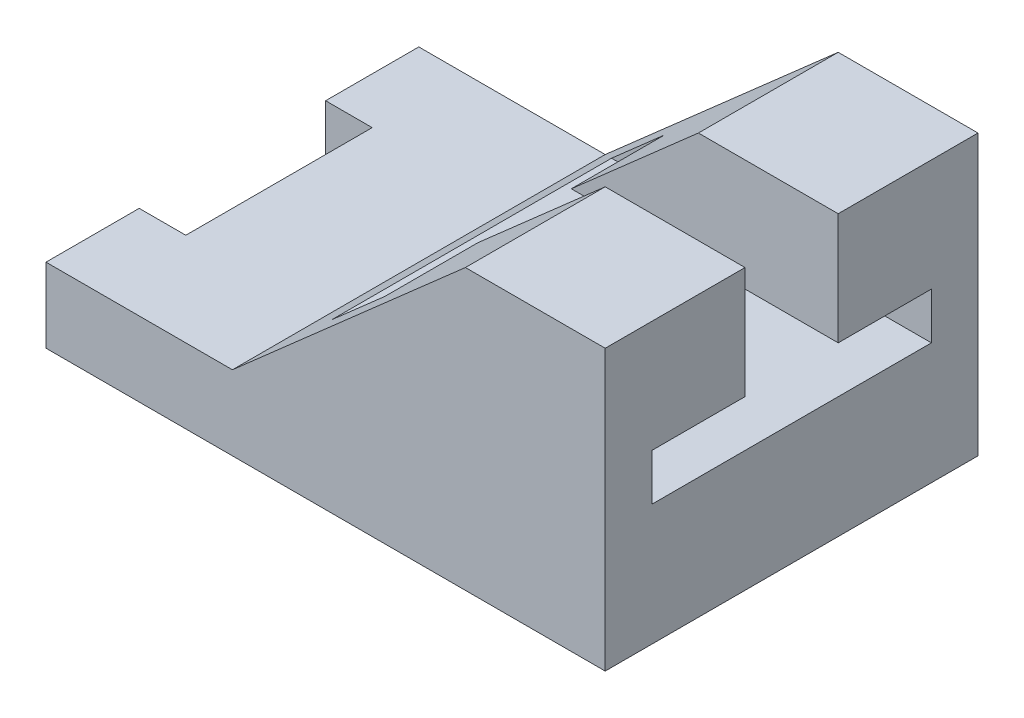
ISO-10303-21;
HEADER;
FILE_DESCRIPTION(('STEP AP214'),'2;1');
FILE_NAME('part.step','',(''),(''),'','','');
FILE_SCHEMA(('AUTOMOTIVE_DESIGN { 1 0 10303 214 1 1 1 1 }'));
ENDSEC;
DATA;
#1=APPLICATION_CONTEXT('core data for automotive mechanical design processes');
#2=APPLICATION_PROTOCOL_DEFINITION('international standard','automotive_design',2000,#1);
#3=PRODUCT_CONTEXT('',#1,'mechanical');
#4=PRODUCT('Part','Part','',(#3));
#5=PRODUCT_RELATED_PRODUCT_CATEGORY('part','',(#4));
#6=PRODUCT_DEFINITION_FORMATION('','',#4);
#7=PRODUCT_DEFINITION_CONTEXT('part definition',#1,'design');
#8=PRODUCT_DEFINITION('design','',#6,#7);
#9=PRODUCT_DEFINITION_SHAPE('','',#8);
#10=(LENGTH_UNIT() NAMED_UNIT(*) SI_UNIT(.MILLI.,.METRE.));
#11=(NAMED_UNIT(*) PLANE_ANGLE_UNIT() SI_UNIT($,.RADIAN.));
#12=(NAMED_UNIT(*) SI_UNIT($,.STERADIAN.) SOLID_ANGLE_UNIT());
#13=UNCERTAINTY_MEASURE_WITH_UNIT(LENGTH_MEASURE(1.E-05),#10,'distance_accuracy_value','');
#14=(GEOMETRIC_REPRESENTATION_CONTEXT(3) GLOBAL_UNCERTAINTY_ASSIGNED_CONTEXT((#13)) GLOBAL_UNIT_ASSIGNED_CONTEXT((#10,
#11,#12)) REPRESENTATION_CONTEXT('',''));
#15=CARTESIAN_POINT('',(0.,0.,0.));
#16=DIRECTION('',(0.,0.,1.));
#17=DIRECTION('',(1.,0.,0.));
#18=AXIS2_PLACEMENT_3D('',#15,#16,#17);
#19=CARTESIAN_POINT('',(60.,30.,40.));
#20=DIRECTION('',(0.,-1.,0.));
#21=DIRECTION('',(0.,0.,-1.));
#22=AXIS2_PLACEMENT_3D('',#19,#20,#21);
#23=PLANE('',#22);
#24=DIRECTION('',(0.,0.,-1.));
#25=VECTOR('',#24,1.);
#26=CARTESIAN_POINT('',(45.,30.,40.));
#27=LINE('',#26,#25);
#28=CARTESIAN_POINT('',(45.,30.,15.));
#29=VERTEX_POINT('',#28);
#30=CARTESIAN_POINT('',(45.,30.,0.));
#31=VERTEX_POINT('',#30);
#32=EDGE_CURVE('E302',#29,#31,#27,.T.);
#33=ORIENTED_EDGE('',*,*,#32,.F.);
#34=DIRECTION('',(1.,0.,0.));
#35=VECTOR('',#34,1.);
#36=CARTESIAN_POINT('',(20.,30.,15.));
#37=LINE('',#36,#35);
#38=CARTESIAN_POINT('',(60.,30.,15.));
#39=VERTEX_POINT('',#38);
#40=EDGE_CURVE('E240',#29,#39,#37,.T.);
#41=ORIENTED_EDGE('',*,*,#40,.T.);
#42=DIRECTION('',(0.,0.,-1.));
#43=VECTOR('',#42,1.);
#44=CARTESIAN_POINT('',(60.,30.,40.));
#45=LINE('',#44,#43);
#46=CARTESIAN_POINT('',(60.,30.,0.));
#47=VERTEX_POINT('',#46);
#48=EDGE_CURVE('E194',#39,#47,#45,.T.);
#49=ORIENTED_EDGE('',*,*,#48,.T.);
#50=DIRECTION('',(-1.,0.,0.));
#51=VECTOR('',#50,1.);
#52=CARTESIAN_POINT('',(60.,30.,0.));
#53=LINE('',#52,#51);
#54=EDGE_CURVE('E292',#47,#31,#53,.T.);
#55=ORIENTED_EDGE('',*,*,#54,.T.);
#56=EDGE_LOOP('',(#33,#41,#49,#55));
#57=FACE_BOUND('',#56,.T.);
#58=ADVANCED_FACE('F43',(#57),#23,.F.);
#59=CARTESIAN_POINT('',(0.,0.,40.));
#60=DIRECTION('',(1.,0.,0.));
#61=DIRECTION('',(0.,0.,-1.));
#62=AXIS2_PLACEMENT_3D('',#59,#60,#61);
#63=PLANE('',#62);
#64=DIRECTION('',(0.,0.,-1.));
#65=VECTOR('',#64,1.);
#66=CARTESIAN_POINT('',(0.,8.,40.));
#67=LINE('',#66,#65);
#68=CARTESIAN_POINT('',(0.,8.,40.));
#69=VERTEX_POINT('',#68);
#70=CARTESIAN_POINT('',(0.,8.,30.));
#71=VERTEX_POINT('',#70);
#72=EDGE_CURVE('E297',#69,#71,#67,.T.);
#73=ORIENTED_EDGE('',*,*,#72,.T.);
#74=DIRECTION('',(0.,1.,0.));
#75=VECTOR('',#74,1.);
#76=CARTESIAN_POINT('',(0.,0.,30.));
#77=LINE('',#76,#75);
#78=CARTESIAN_POINT('',(0.,0.,30.));
#79=VERTEX_POINT('',#78);
#80=EDGE_CURVE('E250',#79,#71,#77,.T.);
#81=ORIENTED_EDGE('',*,*,#80,.F.);
#82=DIRECTION('',(0.,0.,-1.));
#83=VECTOR('',#82,1.);
#84=CARTESIAN_POINT('',(0.,0.,40.));
#85=LINE('',#84,#83);
#86=CARTESIAN_POINT('',(0.,0.,40.));
#87=VERTEX_POINT('',#86);
#88=EDGE_CURVE('E205',#87,#79,#85,.T.);
#89=ORIENTED_EDGE('',*,*,#88,.F.);
#90=DIRECTION('',(0.,-1.,0.));
#91=VECTOR('',#90,1.);
#92=CARTESIAN_POINT('',(0.,0.,40.));
#93=LINE('',#92,#91);
#94=EDGE_CURVE('E269',#69,#87,#93,.T.);
#95=ORIENTED_EDGE('',*,*,#94,.F.);
#96=EDGE_LOOP('',(#73,#81,#89,#95));
#97=FACE_BOUND('',#96,.T.);
#98=ADVANCED_FACE('F352',(#97),#63,.F.);
#99=CARTESIAN_POINT('',(0.,0.,10.));
#100=VERTEX_POINT('',#99);
#101=CARTESIAN_POINT('',(0.,0.,0.));
#102=VERTEX_POINT('',#101);
#103=EDGE_CURVE('E198',#100,#102,#85,.T.);
#104=ORIENTED_EDGE('',*,*,#103,.F.);
#105=DIRECTION('',(0.,-1.,0.));
#106=VECTOR('',#105,1.);
#107=CARTESIAN_POINT('',(0.,8.,10.));
#108=LINE('',#107,#106);
#109=CARTESIAN_POINT('',(0.,8.,10.));
#110=VERTEX_POINT('',#109);
#111=EDGE_CURVE('E260',#110,#100,#108,.T.);
#112=ORIENTED_EDGE('',*,*,#111,.F.);
#113=CARTESIAN_POINT('',(0.,8.,0.));
#114=VERTEX_POINT('',#113);
#115=EDGE_CURVE('E282',#110,#114,#67,.T.);
#116=ORIENTED_EDGE('',*,*,#115,.T.);
#117=DIRECTION('',(0.,-1.,0.));
#118=VECTOR('',#117,1.);
#119=CARTESIAN_POINT('',(0.,0.,0.));
#120=LINE('',#119,#118);
#121=EDGE_CURVE('E263',#114,#102,#120,.T.);
#122=ORIENTED_EDGE('',*,*,#121,.T.);
#123=EDGE_LOOP('',(#104,#112,#116,#122));
#124=FACE_BOUND('',#123,.T.);
#125=ADVANCED_FACE('F44',(#124),#63,.F.);
#126=CARTESIAN_POINT('',(0.,0.,40.));
#127=DIRECTION('',(0.,1.,0.));
#128=DIRECTION('',(0.,0.,1.));
#129=AXIS2_PLACEMENT_3D('',#126,#127,#128);
#130=PLANE('',#129);
#131=ORIENTED_EDGE('',*,*,#88,.T.);
#132=DIRECTION('',(-1.,0.,0.));
#133=VECTOR('',#132,1.);
#134=CARTESIAN_POINT('',(5.,0.,30.));
#135=LINE('',#134,#133);
#136=CARTESIAN_POINT('',(5.,0.,30.));
#137=VERTEX_POINT('',#136);
#138=EDGE_CURVE('E262',#137,#79,#135,.T.);
#139=ORIENTED_EDGE('',*,*,#138,.F.);
#140=DIRECTION('',(0.,0.,1.));
#141=VECTOR('',#140,1.);
#142=CARTESIAN_POINT('',(5.,0.,10.));
#143=LINE('',#142,#141);
#144=CARTESIAN_POINT('',(5.,0.,10.));
#145=VERTEX_POINT('',#144);
#146=EDGE_CURVE('E251',#145,#137,#143,.T.);
#147=ORIENTED_EDGE('',*,*,#146,.F.);
#148=DIRECTION('',(-1.,0.,0.));
#149=VECTOR('',#148,1.);
#150=CARTESIAN_POINT('',(5.,0.,10.));
#151=LINE('',#150,#149);
#152=EDGE_CURVE('E266',#145,#100,#151,.T.);
#153=ORIENTED_EDGE('',*,*,#152,.T.);
#154=ORIENTED_EDGE('',*,*,#103,.T.);
#155=DIRECTION('',(1.,0.,0.));
#156=VECTOR('',#155,1.);
#157=CARTESIAN_POINT('',(0.,0.,0.));
#158=LINE('',#157,#156);
#159=CARTESIAN_POINT('',(60.,0.,0.));
#160=VERTEX_POINT('',#159);
#161=EDGE_CURVE('E286',#102,#160,#158,.T.);
#162=ORIENTED_EDGE('',*,*,#161,.T.);
#163=DIRECTION('',(0.,0.,-1.));
#164=VECTOR('',#163,1.);
#165=CARTESIAN_POINT('',(60.,0.,40.));
#166=LINE('',#165,#164);
#167=CARTESIAN_POINT('',(60.,0.,40.));
#168=VERTEX_POINT('',#167);
#169=EDGE_CURVE('E192',#168,#160,#166,.T.);
#170=ORIENTED_EDGE('',*,*,#169,.F.);
#171=DIRECTION('',(1.,0.,0.));
#172=VECTOR('',#171,1.);
#173=CARTESIAN_POINT('',(0.,0.,40.));
#174=LINE('',#173,#172);
#175=EDGE_CURVE('E272',#87,#168,#174,.T.);
#176=ORIENTED_EDGE('',*,*,#175,.F.);
#177=EDGE_LOOP('',(#131,#139,#147,#153,#154,#162,#170,#176));
#178=FACE_BOUND('',#177,.T.);
#179=ADVANCED_FACE('F370',(#178),#130,.F.);
#180=CARTESIAN_POINT('',(60.,0.,40.));
#181=DIRECTION('',(-1.,0.,0.));
#182=DIRECTION('',(0.,0.,1.));
#183=AXIS2_PLACEMENT_3D('',#180,#181,#182);
#184=PLANE('',#183);
#185=ORIENTED_EDGE('',*,*,#48,.F.);
#186=DIRECTION('',(0.,1.,0.));
#187=VECTOR('',#186,1.);
#188=CARTESIAN_POINT('',(60.,30.,15.));
#189=LINE('',#188,#187);
#190=CARTESIAN_POINT('',(60.,18.,15.));
#191=VERTEX_POINT('',#190);
#192=EDGE_CURVE('E177',#191,#39,#189,.T.);
#193=ORIENTED_EDGE('',*,*,#192,.F.);
#194=DIRECTION('',(0.,0.,1.));
#195=VECTOR('',#194,1.);
#196=CARTESIAN_POINT('',(60.,18.,15.));
#197=LINE('',#196,#195);
#198=CARTESIAN_POINT('',(60.,18.,5.));
#199=VERTEX_POINT('',#198);
#200=EDGE_CURVE('E323',#199,#191,#197,.T.);
#201=ORIENTED_EDGE('',*,*,#200,.F.);
#202=DIRECTION('',(0.,1.,0.));
#203=VECTOR('',#202,1.);
#204=CARTESIAN_POINT('',(60.,18.,5.));
#205=LINE('',#204,#203);
#206=CARTESIAN_POINT('',(60.,13.,5.));
#207=VERTEX_POINT('',#206);
#208=EDGE_CURVE('E234',#207,#199,#205,.T.);
#209=ORIENTED_EDGE('',*,*,#208,.F.);
#210=DIRECTION('',(0.,0.,-1.));
#211=VECTOR('',#210,1.);
#212=CARTESIAN_POINT('',(60.,13.,5.));
#213=LINE('',#212,#211);
#214=CARTESIAN_POINT('',(60.,13.,35.));
#215=VERTEX_POINT('',#214);
#216=EDGE_CURVE('E328',#215,#207,#213,.T.);
#217=ORIENTED_EDGE('',*,*,#216,.F.);
#218=DIRECTION('',(0.,-1.,0.));
#219=VECTOR('',#218,1.);
#220=CARTESIAN_POINT('',(60.,13.,35.));
#221=LINE('',#220,#219);
#222=CARTESIAN_POINT('',(60.,18.,35.));
#223=VERTEX_POINT('',#222);
#224=EDGE_CURVE('E335',#223,#215,#221,.T.);
#225=ORIENTED_EDGE('',*,*,#224,.F.);
#226=DIRECTION('',(0.,0.,1.));
#227=VECTOR('',#226,1.);
#228=CARTESIAN_POINT('',(60.,18.,35.));
#229=LINE('',#228,#227);
#230=CARTESIAN_POINT('',(60.,18.,25.));
#231=VERTEX_POINT('',#230);
#232=EDGE_CURVE('E187',#231,#223,#229,.T.);
#233=ORIENTED_EDGE('',*,*,#232,.F.);
#234=DIRECTION('',(0.,-1.,0.));
#235=VECTOR('',#234,1.);
#236=CARTESIAN_POINT('',(60.,30.,25.));
#237=LINE('',#236,#235);
#238=CARTESIAN_POINT('',(60.,30.,25.));
#239=VERTEX_POINT('',#238);
#240=EDGE_CURVE('E166',#239,#231,#237,.T.);
#241=ORIENTED_EDGE('',*,*,#240,.F.);
#242=CARTESIAN_POINT('',(60.,30.,40.));
#243=VERTEX_POINT('',#242);
#244=EDGE_CURVE('E184',#243,#239,#45,.T.);
#245=ORIENTED_EDGE('',*,*,#244,.F.);
#246=DIRECTION('',(0.,1.,0.));
#247=VECTOR('',#246,1.);
#248=CARTESIAN_POINT('',(60.,0.,40.));
#249=LINE('',#248,#247);
#250=EDGE_CURVE('E277',#168,#243,#249,.T.);
#251=ORIENTED_EDGE('',*,*,#250,.F.);
#252=ORIENTED_EDGE('',*,*,#169,.T.);
#253=DIRECTION('',(0.,1.,0.));
#254=VECTOR('',#253,1.);
#255=CARTESIAN_POINT('',(60.,0.,0.));
#256=LINE('',#255,#254);
#257=EDGE_CURVE('E289',#160,#47,#256,.T.);
#258=ORIENTED_EDGE('',*,*,#257,.T.);
#259=EDGE_LOOP('',(#185,#193,#201,#209,#217,#225,#233,#241,#245,#251,#252,#258));
#260=FACE_BOUND('',#259,.T.);
#261=ADVANCED_FACE('F185',(#260),#184,.F.);
#262=ORIENTED_EDGE('',*,*,#244,.T.);
#263=DIRECTION('',(1.,0.,0.));
#264=VECTOR('',#263,1.);
#265=CARTESIAN_POINT('',(20.,30.,25.));
#266=LINE('',#265,#264);
#267=CARTESIAN_POINT('',(45.,30.,25.));
#268=VERTEX_POINT('',#267);
#269=EDGE_CURVE('E167',#268,#239,#266,.T.);
#270=ORIENTED_EDGE('',*,*,#269,.F.);
#271=CARTESIAN_POINT('',(45.,30.,40.));
#272=VERTEX_POINT('',#271);
#273=EDGE_CURVE('E196',#272,#268,#27,.T.);
#274=ORIENTED_EDGE('',*,*,#273,.F.);
#275=DIRECTION('',(-1.,0.,0.));
#276=VECTOR('',#275,1.);
#277=CARTESIAN_POINT('',(60.,30.,40.));
#278=LINE('',#277,#276);
#279=EDGE_CURVE('E191',#243,#272,#278,.T.);
#280=ORIENTED_EDGE('',*,*,#279,.F.);
#281=EDGE_LOOP('',(#262,#270,#274,#280));
#282=FACE_BOUND('',#281,.T.);
#283=ADVANCED_FACE('F186',(#282),#23,.F.);
#284=CARTESIAN_POINT('',(20.,8.,40.));
#285=DIRECTION('',(0.660627894892025,-0.750713516922755,0.));
#286=DIRECTION('',(0.750713516922755,0.660627894892025,0.));
#287=AXIS2_PLACEMENT_3D('',#284,#285,#286);
#288=PLANE('',#287);
#289=DIRECTION('',(0.,0.,1.));
#290=VECTOR('',#289,1.);
#291=CARTESIAN_POINT('',(31.3636363636364,18.,40.));
#292=LINE('',#291,#290);
#293=CARTESIAN_POINT('',(31.3636363636364,18.,5.));
#294=VERTEX_POINT('',#293);
#295=CARTESIAN_POINT('',(31.3636363636364,18.,15.));
#296=VERTEX_POINT('',#295);
#297=EDGE_CURVE('E51',#294,#296,#292,.T.);
#298=ORIENTED_EDGE('',*,*,#297,.T.);
#299=DIRECTION('',(0.750713516922755,0.660627894892025,0.));
#300=VECTOR('',#299,1.);
#301=CARTESIAN_POINT('',(20.,8.,15.));
#302=LINE('',#301,#300);
#303=EDGE_CURVE('E11',#296,#29,#302,.T.);
#304=ORIENTED_EDGE('',*,*,#303,.T.);
#305=ORIENTED_EDGE('',*,*,#32,.T.);
#306=DIRECTION('',(-0.750713516922755,-0.660627894892025,0.));
#307=VECTOR('',#306,1.);
#308=CARTESIAN_POINT('',(20.,8.,0.));
#309=LINE('',#308,#307);
#310=CARTESIAN_POINT('',(20.,8.,0.));
#311=VERTEX_POINT('',#310);
#312=EDGE_CURVE('E294',#31,#311,#309,.T.);
#313=ORIENTED_EDGE('',*,*,#312,.T.);
#314=DIRECTION('',(0.,0.,-1.));
#315=VECTOR('',#314,1.);
#316=CARTESIAN_POINT('',(20.,8.,40.));
#317=LINE('',#316,#315);
#318=CARTESIAN_POINT('',(20.,8.,40.));
#319=VERTEX_POINT('',#318);
#320=EDGE_CURVE('E296',#319,#311,#317,.T.);
#321=ORIENTED_EDGE('',*,*,#320,.F.);
#322=DIRECTION('',(-0.750713516922755,-0.660627894892025,0.));
#323=VECTOR('',#322,1.);
#324=CARTESIAN_POINT('',(20.,8.,40.));
#325=LINE('',#324,#323);
#326=EDGE_CURVE('E276',#272,#319,#325,.T.);
#327=ORIENTED_EDGE('',*,*,#326,.F.);
#328=ORIENTED_EDGE('',*,*,#273,.T.);
#329=DIRECTION('',(-0.750713516922755,-0.660627894892025,0.));
#330=VECTOR('',#329,1.);
#331=CARTESIAN_POINT('',(20.,8.,25.));
#332=LINE('',#331,#330);
#333=CARTESIAN_POINT('',(31.3636363636364,18.,25.));
#334=VERTEX_POINT('',#333);
#335=EDGE_CURVE('E174',#268,#334,#332,.T.);
#336=ORIENTED_EDGE('',*,*,#335,.T.);
#337=DIRECTION('',(0.,0.,1.));
#338=VECTOR('',#337,1.);
#339=CARTESIAN_POINT('',(31.3636363636364,18.,40.));
#340=LINE('',#339,#338);
#341=CARTESIAN_POINT('',(31.3636363636364,18.,35.));
#342=VERTEX_POINT('',#341);
#343=EDGE_CURVE('E206',#334,#342,#340,.T.);
#344=ORIENTED_EDGE('',*,*,#343,.T.);
#345=DIRECTION('',(-0.750713516922755,-0.660627894892025,0.));
#346=VECTOR('',#345,1.);
#347=CARTESIAN_POINT('',(20.,8.,35.));
#348=LINE('',#347,#346);
#349=CARTESIAN_POINT('',(25.6818181818182,13.,35.));
#350=VERTEX_POINT('',#349);
#351=EDGE_CURVE('E207',#342,#350,#348,.T.);
#352=ORIENTED_EDGE('',*,*,#351,.T.);
#353=DIRECTION('',(0.,0.,-1.));
#354=VECTOR('',#353,1.);
#355=CARTESIAN_POINT('',(25.6818181818182,13.,40.));
#356=LINE('',#355,#354);
#357=CARTESIAN_POINT('',(25.6818181818182,13.,5.));
#358=VERTEX_POINT('',#357);
#359=EDGE_CURVE('E215',#350,#358,#356,.T.);
#360=ORIENTED_EDGE('',*,*,#359,.T.);
#361=DIRECTION('',(0.750713516922755,0.660627894892025,0.));
#362=VECTOR('',#361,1.);
#363=CARTESIAN_POINT('',(20.,8.,5.));
#364=LINE('',#363,#362);
#365=EDGE_CURVE('E214',#358,#294,#364,.T.);
#366=ORIENTED_EDGE('',*,*,#365,.T.);
#367=EDGE_LOOP('',(#298,#304,#305,#313,#321,#327,#328,#336,#344,#352,#360,#366));
#368=FACE_BOUND('',#367,.T.);
#369=ADVANCED_FACE('F218',(#368),#288,.F.);
#370=CARTESIAN_POINT('',(0.,8.,40.));
#371=DIRECTION('',(0.,-1.,0.));
#372=DIRECTION('',(0.,0.,-1.));
#373=AXIS2_PLACEMENT_3D('',#370,#371,#372);
#374=PLANE('',#373);
#375=DIRECTION('',(0.,0.,-1.));
#376=VECTOR('',#375,1.);
#377=CARTESIAN_POINT('',(5.,8.,30.));
#378=LINE('',#377,#376);
#379=CARTESIAN_POINT('',(5.,8.,30.));
#380=VERTEX_POINT('',#379);
#381=CARTESIAN_POINT('',(5.,8.,10.));
#382=VERTEX_POINT('',#381);
#383=EDGE_CURVE('E247',#380,#382,#378,.T.);
#384=ORIENTED_EDGE('',*,*,#383,.F.);
#385=DIRECTION('',(-1.,0.,0.));
#386=VECTOR('',#385,1.);
#387=CARTESIAN_POINT('',(5.,8.,30.));
#388=LINE('',#387,#386);
#389=EDGE_CURVE('E257',#380,#71,#388,.T.);
#390=ORIENTED_EDGE('',*,*,#389,.T.);
#391=ORIENTED_EDGE('',*,*,#72,.F.);
#392=DIRECTION('',(-1.,0.,0.));
#393=VECTOR('',#392,1.);
#394=CARTESIAN_POINT('',(0.,8.,40.));
#395=LINE('',#394,#393);
#396=EDGE_CURVE('E283',#319,#69,#395,.T.);
#397=ORIENTED_EDGE('',*,*,#396,.F.);
#398=ORIENTED_EDGE('',*,*,#320,.T.);
#399=DIRECTION('',(-1.,0.,0.));
#400=VECTOR('',#399,1.);
#401=CARTESIAN_POINT('',(0.,8.,0.));
#402=LINE('',#401,#400);
#403=EDGE_CURVE('E273',#311,#114,#402,.T.);
#404=ORIENTED_EDGE('',*,*,#403,.T.);
#405=ORIENTED_EDGE('',*,*,#115,.F.);
#406=DIRECTION('',(-1.,0.,0.));
#407=VECTOR('',#406,1.);
#408=CARTESIAN_POINT('',(5.,8.,10.));
#409=LINE('',#408,#407);
#410=EDGE_CURVE('E258',#382,#110,#409,.T.);
#411=ORIENTED_EDGE('',*,*,#410,.F.);
#412=EDGE_LOOP('',(#384,#390,#391,#397,#398,#404,#405,#411));
#413=FACE_BOUND('',#412,.T.);
#414=ADVANCED_FACE('F368',(#413),#374,.F.);
#415=CARTESIAN_POINT('',(0.,0.,40.));
#416=DIRECTION('',(0.,0.,-1.));
#417=DIRECTION('',(-1.,0.,0.));
#418=AXIS2_PLACEMENT_3D('',#415,#416,#417);
#419=PLANE('',#418);
#420=ORIENTED_EDGE('',*,*,#94,.T.);
#421=ORIENTED_EDGE('',*,*,#175,.T.);
#422=ORIENTED_EDGE('',*,*,#250,.T.);
#423=ORIENTED_EDGE('',*,*,#279,.T.);
#424=ORIENTED_EDGE('',*,*,#326,.T.);
#425=ORIENTED_EDGE('',*,*,#396,.T.);
#426=EDGE_LOOP('',(#420,#421,#422,#423,#424,#425));
#427=FACE_BOUND('',#426,.T.);
#428=ADVANCED_FACE('F310',(#427),#419,.F.);
#429=CARTESIAN_POINT('',(0.,0.,0.));
#430=DIRECTION('',(0.,0.,-1.));
#431=DIRECTION('',(-1.,0.,0.));
#432=AXIS2_PLACEMENT_3D('',#429,#430,#431);
#433=PLANE('',#432);
#434=ORIENTED_EDGE('',*,*,#121,.F.);
#435=ORIENTED_EDGE('',*,*,#403,.F.);
#436=ORIENTED_EDGE('',*,*,#312,.F.);
#437=ORIENTED_EDGE('',*,*,#54,.F.);
#438=ORIENTED_EDGE('',*,*,#257,.F.);
#439=ORIENTED_EDGE('',*,*,#161,.F.);
#440=EDGE_LOOP('',(#434,#435,#436,#437,#438,#439));
#441=FACE_BOUND('',#440,.T.);
#442=ADVANCED_FACE('F318',(#441),#433,.T.);
#443=CARTESIAN_POINT('',(5.,0.,30.));
#444=DIRECTION('',(0.,0.,1.));
#445=DIRECTION('',(1.,0.,0.));
#446=AXIS2_PLACEMENT_3D('',#443,#444,#445);
#447=PLANE('',#446);
#448=ORIENTED_EDGE('',*,*,#80,.T.);
#449=ORIENTED_EDGE('',*,*,#389,.F.);
#450=DIRECTION('',(0.,1.,0.));
#451=VECTOR('',#450,1.);
#452=CARTESIAN_POINT('',(5.,0.,30.));
#453=LINE('',#452,#451);
#454=EDGE_CURVE('E66',#137,#380,#453,.T.);
#455=ORIENTED_EDGE('',*,*,#454,.F.);
#456=ORIENTED_EDGE('',*,*,#138,.T.);
#457=EDGE_LOOP('',(#448,#449,#455,#456));
#458=FACE_BOUND('',#457,.T.);
#459=ADVANCED_FACE('F381',(#458),#447,.F.);
#460=CARTESIAN_POINT('',(5.,8.,10.));
#461=DIRECTION('',(0.,0.,-1.));
#462=DIRECTION('',(-1.,0.,0.));
#463=AXIS2_PLACEMENT_3D('',#460,#461,#462);
#464=PLANE('',#463);
#465=ORIENTED_EDGE('',*,*,#111,.T.);
#466=ORIENTED_EDGE('',*,*,#152,.F.);
#467=DIRECTION('',(0.,-1.,0.));
#468=VECTOR('',#467,1.);
#469=CARTESIAN_POINT('',(5.,8.,10.));
#470=LINE('',#469,#468);
#471=EDGE_CURVE('E248',#382,#145,#470,.T.);
#472=ORIENTED_EDGE('',*,*,#471,.F.);
#473=ORIENTED_EDGE('',*,*,#410,.T.);
#474=EDGE_LOOP('',(#465,#466,#472,#473));
#475=FACE_BOUND('',#474,.T.);
#476=ADVANCED_FACE('F389',(#475),#464,.F.);
#477=CARTESIAN_POINT('',(5.,0.,0.));
#478=DIRECTION('',(-1.,0.,0.));
#479=DIRECTION('',(0.,0.,1.));
#480=AXIS2_PLACEMENT_3D('',#477,#478,#479);
#481=PLANE('',#480);
#482=ORIENTED_EDGE('',*,*,#383,.T.);
#483=ORIENTED_EDGE('',*,*,#471,.T.);
#484=ORIENTED_EDGE('',*,*,#146,.T.);
#485=ORIENTED_EDGE('',*,*,#454,.T.);
#486=EDGE_LOOP('',(#482,#483,#484,#485));
#487=FACE_BOUND('',#486,.T.);
#488=ADVANCED_FACE('F387',(#487),#481,.T.);
#489=CARTESIAN_POINT('',(20.,30.,15.));
#490=DIRECTION('',(0.,0.,-1.));
#491=DIRECTION('',(-1.,0.,0.));
#492=AXIS2_PLACEMENT_3D('',#489,#490,#491);
#493=PLANE('',#492);
#494=DIRECTION('',(1.,0.,0.));
#495=VECTOR('',#494,1.);
#496=CARTESIAN_POINT('',(20.,18.,15.));
#497=LINE('',#496,#495);
#498=EDGE_CURVE('E227',#296,#191,#497,.T.);
#499=ORIENTED_EDGE('',*,*,#498,.T.);
#500=ORIENTED_EDGE('',*,*,#192,.T.);
#501=ORIENTED_EDGE('',*,*,#40,.F.);
#502=ORIENTED_EDGE('',*,*,#303,.F.);
#503=EDGE_LOOP('',(#499,#500,#501,#502));
#504=FACE_BOUND('',#503,.T.);
#505=ADVANCED_FACE('F397',(#504),#493,.F.);
#506=CARTESIAN_POINT('',(20.,18.,15.));
#507=DIRECTION('',(0.,1.,0.));
#508=DIRECTION('',(0.,0.,1.));
#509=AXIS2_PLACEMENT_3D('',#506,#507,#508);
#510=PLANE('',#509);
#511=DIRECTION('',(1.,0.,0.));
#512=VECTOR('',#511,1.);
#513=CARTESIAN_POINT('',(20.,18.,5.));
#514=LINE('',#513,#512);
#515=EDGE_CURVE('E228',#294,#199,#514,.T.);
#516=ORIENTED_EDGE('',*,*,#515,.T.);
#517=ORIENTED_EDGE('',*,*,#200,.T.);
#518=ORIENTED_EDGE('',*,*,#498,.F.);
#519=ORIENTED_EDGE('',*,*,#297,.F.);
#520=EDGE_LOOP('',(#516,#517,#518,#519));
#521=FACE_BOUND('',#520,.T.);
#522=ADVANCED_FACE('F221',(#521),#510,.F.);
#523=CARTESIAN_POINT('',(20.,18.,5.));
#524=DIRECTION('',(0.,0.,-1.));
#525=DIRECTION('',(-1.,0.,0.));
#526=AXIS2_PLACEMENT_3D('',#523,#524,#525);
#527=PLANE('',#526);
#528=DIRECTION('',(1.,0.,0.));
#529=VECTOR('',#528,1.);
#530=CARTESIAN_POINT('',(20.,13.,5.));
#531=LINE('',#530,#529);
#532=EDGE_CURVE('E235',#358,#207,#531,.T.);
#533=ORIENTED_EDGE('',*,*,#532,.T.);
#534=ORIENTED_EDGE('',*,*,#208,.T.);
#535=ORIENTED_EDGE('',*,*,#515,.F.);
#536=ORIENTED_EDGE('',*,*,#365,.F.);
#537=EDGE_LOOP('',(#533,#534,#535,#536));
#538=FACE_BOUND('',#537,.T.);
#539=ADVANCED_FACE('F226',(#538),#527,.F.);
#540=CARTESIAN_POINT('',(20.,13.,5.));
#541=DIRECTION('',(0.,-1.,0.));
#542=DIRECTION('',(0.,0.,-1.));
#543=AXIS2_PLACEMENT_3D('',#540,#541,#542);
#544=PLANE('',#543);
#545=DIRECTION('',(1.,0.,0.));
#546=VECTOR('',#545,1.);
#547=CARTESIAN_POINT('',(20.,13.,35.));
#548=LINE('',#547,#546);
#549=EDGE_CURVE('E239',#350,#215,#548,.T.);
#550=ORIENTED_EDGE('',*,*,#549,.T.);
#551=ORIENTED_EDGE('',*,*,#216,.T.);
#552=ORIENTED_EDGE('',*,*,#532,.F.);
#553=ORIENTED_EDGE('',*,*,#359,.F.);
#554=EDGE_LOOP('',(#550,#551,#552,#553));
#555=FACE_BOUND('',#554,.T.);
#556=ADVANCED_FACE('F344',(#555),#544,.F.);
#557=CARTESIAN_POINT('',(20.,13.,35.));
#558=DIRECTION('',(0.,0.,1.));
#559=DIRECTION('',(1.,0.,0.));
#560=AXIS2_PLACEMENT_3D('',#557,#558,#559);
#561=PLANE('',#560);
#562=DIRECTION('',(1.,0.,0.));
#563=VECTOR('',#562,1.);
#564=CARTESIAN_POINT('',(20.,18.,35.));
#565=LINE('',#564,#563);
#566=EDGE_CURVE('E245',#342,#223,#565,.T.);
#567=ORIENTED_EDGE('',*,*,#566,.T.);
#568=ORIENTED_EDGE('',*,*,#224,.T.);
#569=ORIENTED_EDGE('',*,*,#549,.F.);
#570=ORIENTED_EDGE('',*,*,#351,.F.);
#571=EDGE_LOOP('',(#567,#568,#569,#570));
#572=FACE_BOUND('',#571,.T.);
#573=ADVANCED_FACE('F341',(#572),#561,.F.);
#574=CARTESIAN_POINT('',(20.,18.,35.));
#575=DIRECTION('',(0.,1.,0.));
#576=DIRECTION('',(0.,0.,1.));
#577=AXIS2_PLACEMENT_3D('',#574,#575,#576);
#578=PLANE('',#577);
#579=DIRECTION('',(1.,0.,0.));
#580=VECTOR('',#579,1.);
#581=CARTESIAN_POINT('',(20.,18.,25.));
#582=LINE('',#581,#580);
#583=EDGE_CURVE('E59',#334,#231,#582,.T.);
#584=ORIENTED_EDGE('',*,*,#583,.T.);
#585=ORIENTED_EDGE('',*,*,#232,.T.);
#586=ORIENTED_EDGE('',*,*,#566,.F.);
#587=ORIENTED_EDGE('',*,*,#343,.F.);
#588=EDGE_LOOP('',(#584,#585,#586,#587));
#589=FACE_BOUND('',#588,.T.);
#590=ADVANCED_FACE('F339',(#589),#578,.F.);
#591=CARTESIAN_POINT('',(20.,30.,25.));
#592=DIRECTION('',(0.,0.,1.));
#593=DIRECTION('',(1.,0.,0.));
#594=AXIS2_PLACEMENT_3D('',#591,#592,#593);
#595=PLANE('',#594);
#596=ORIENTED_EDGE('',*,*,#269,.T.);
#597=ORIENTED_EDGE('',*,*,#240,.T.);
#598=ORIENTED_EDGE('',*,*,#583,.F.);
#599=ORIENTED_EDGE('',*,*,#335,.F.);
#600=EDGE_LOOP('',(#596,#597,#598,#599));
#601=FACE_BOUND('',#600,.T.);
#602=ADVANCED_FACE('F169',(#601),#595,.F.);
#603=CLOSED_SHELL('',(#58,#98,#125,#179,#261,#283,#369,#414,#428,#442,#459,#476,#488,#505,#522,
#539,#556,#573,#590,#602));
#604=MANIFOLD_SOLID_BREP('B2',#603);
#605=ADVANCED_BREP_SHAPE_REPRESENTATION('',(#18,#604),#14);
#606=SHAPE_DEFINITION_REPRESENTATION(#9,#605);
ENDSEC;
END-ISO-10303-21;
